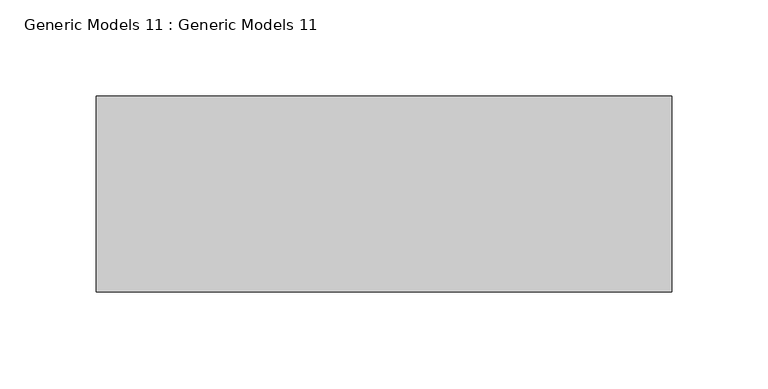
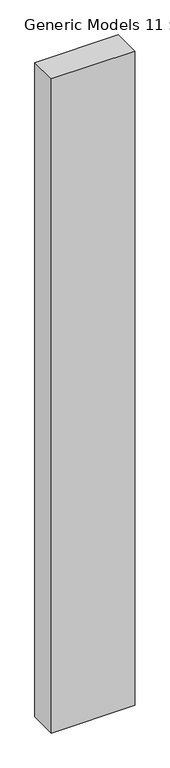
"""IFC4 building model written with IfcOpenShell, lengths in millimetres: proxy geometry, Generic Models 11 : Generic Models 11."""

from ifc_helpers import new_model, si_unit, frame, origin, place, context, project, spatial, polyline, outline, extrude, source, transform, mapped, element, save


def generic_models_11_generic_models_11_c52e9c8d(model_context):
    return source(origin(), model_context, "Body", "SweptSolid", [
        extrude(outline(polyline([(-1047.5736584, -10390.4050402), (-1346.0236584, -10390.4050402), (-1346.0236584, -10288.8050402), (-1047.5736584, -10288.8050402), (-1047.5736584, -10390.4050402)])), frame((0.0, 0.0, 304.8), z_axis=(0.0, 0.0, 1.0), x_axis=(1.0, 0.0, 0.0)), (0.0, 0.0, 1.0), 2476.5),
    ])


if __name__ == "__main__":
    model = new_model("IFC4")
    model_context = context("Model", 3, world=origin())
    ifc_project = project(units=[si_unit("LENGTHUNIT", "METRE", prefix="MILLI")], contexts=[model_context])
    site = spatial("IfcSite", under=ifc_project)
    building = spatial("IfcBuilding", under=site)
    placement = place(None, origin())
    generic_models_11_generic_models_11_shape = generic_models_11_generic_models_11_c52e9c8d(model_context)
    element("IfcBuildingElementProxy", 1, Name="Generic Models 11 : Generic Models 11", ObjectType="Generic Models 11 : Generic Models 11", at=placement, inside=building, context=model_context, shape_type="MappedRepresentation", body=[
        mapped(generic_models_11_generic_models_11_shape, transform((0.0, 0.0, 0.0), x_axis=(1.0, 0.0, 0.0), y_axis=(0.0, 1.0, 0.0), z_axis=(0.0, 0.0, 1.0))),
    ])
    save(model, "model.ifc")

# Revit data of these elements
# Element 1 (IfcBuildingElementProxy, "Generic Models 11 : Generic Models 11")
#   Materials on its faces: "ACCENT BEIGE COLOUR"
# Materials
#   "ACCENT BEIGE COLOUR": class "Generic", colour RGB 120 120 120, transparency 0, Cost = 0
